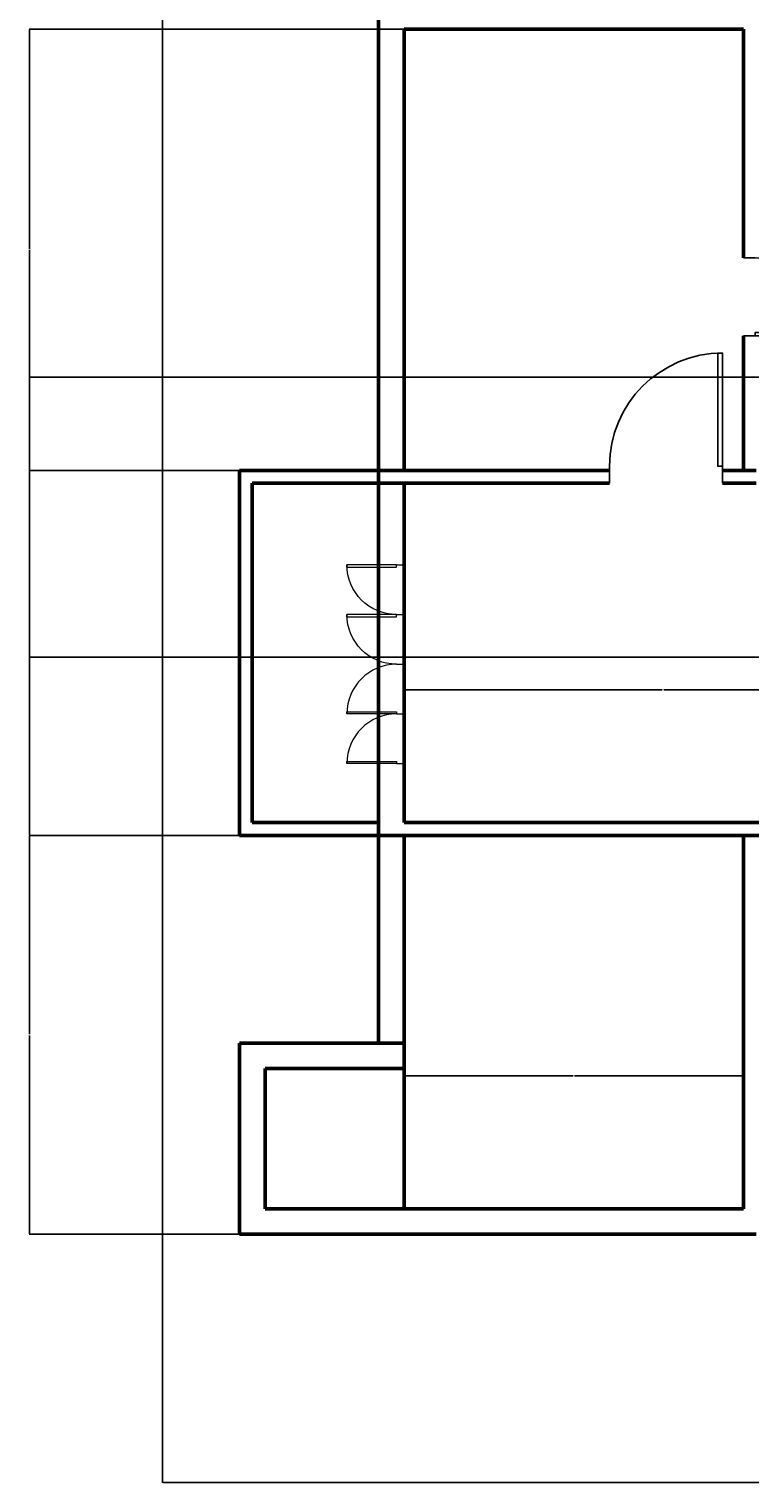
# Model space of a CAD drawing. Units: inches. Extents: x 2032 to 3981, y 840 to 2177.
# Tile 1 of 6: x 2032 to 2286, y 840 to 1354. Entities that reach past the tile are written whole.
import ezdxf

# ---------------------------------------------------------------- set-up
doc = ezdxf.new("R2010")
doc.units = ezdxf.units.IN
for name, color, linetype, lineweight in [('A-ANNO-DIMS', 2, 'Continuous', 18), ('A-DOOR', 3, 'Continuous', 25), ('A-GLAZ', 4, 'Continuous', 18), ('A-WALL', 7, 'Continuous', 50)]:
    doc.layers.add(name, color=color, linetype=linetype, lineweight=lineweight)
doc.styles.get("Standard").update_dxf_attribs({"font": 'arial.ttf'})
doc.dimstyles.get("Standard").update_dxf_attribs({"dimtxt": 0.18, "dimasz": 0.18, "dimexe": 0.18, "dimexo": 0.0625, "dimgap": 0.09, "dimtad": 0, "dimtih": 1, "dimtoh": 1, "dimdec": 4, "dimzin": 0, "dimdsep": 46, "dimtxsty": 'Standard', "dimcen": 0.09, "dimadec": 0, "dimazin": 0, "dimtfac": 1, "dimtdec": 4, "dimtofl": 0, "dimtmove": 0, "dimatfit": 3, "dimfxl": 1, "dimtolj": 1, "dimtzin": 0, "dimarcsym": 0})

# ---------------------------------------------------------------- blocks, each defined once
blk = doc.blocks.new('*U2')
for p, q in [((0, 0), (0, -6)), ((40, 0), (40, -6))]:
    blk.add_line(p, q)
blk.add_lwpolyline([(0, 0), (0, 40), (1.75, 40), (1.75, 0)], close=True)
blk.add_arc((0, 0), 40, 0, 90)
blk = doc.blocks.new('*D14')
at = {"layer": 'A-ANNO-DIMS', "color": 0, "lineweight": -2, "transparency": 16777216}
for p, q in [((2078.89, 1518.9), (2078.89, 840.08)), ((2677.35, 1476.9), (2677.35, 840.08)), ((2079.07, 840.26), (2377.73, 840.26)), ((2677.17, 840.26), (2378.52, 840.26))]:
    blk.add_line(p, q, dxfattribs=at)
at = {"layer": 'A-ANNO-DIMS', "color": 0, "lineweight": 100, "transparency": 16777216}
for points in [[(2079.07, 840.29), (2079.07, 840.23), (2078.89, 840.26)], [(2677.17, 840.29), (2677.17, 840.23), (2677.35, 840.26)]]:
    blk.add_solid(points, dxfattribs=at)
at = {"layer": 'Defpoints', "color": 0, "lineweight": 100, "transparency": 16777216}
for p in [(2078.89, 1518.96), (2677.35, 1476.96), (2677.35, 840.26)]:
    blk.add_point(p, dxfattribs=at)
at = {"layer": 'A-ANNO-DIMS', "color": 0, "transparency": 16777216, "insert": (2378.12, 840.26), "char_height": 0.18, "attachment_point": 5}
blk.add_mtext('\\A1;598.5', dxfattribs=at)
blk = doc.blocks.new('*D22')
at = {"layer": 'A-ANNO-DIMS', "color": 0, "lineweight": -2, "transparency": 16777216}
for p, q in [((2106.03, 1068.96), (2031.71, 1068.96)), ((2031.89, 1068.78), (2031.89, 998.64)), ((2031.89, 928.14), (2031.89, 998.28)), ((2106.03, 927.96), (2031.71, 927.96))]:
    blk.add_line(p, q, dxfattribs=at)
at = {"layer": 'A-ANNO-DIMS', "color": 0, "lineweight": 100, "transparency": 16777216}
for points in [[(2031.86, 1068.78), (2031.92, 1068.78), (2031.89, 1068.96)], [(2031.86, 928.14), (2031.92, 928.14), (2031.89, 927.96)]]:
    blk.add_solid(points, dxfattribs=at)
at = {"layer": 'Defpoints', "color": 0, "lineweight": 100, "transparency": 16777216}
for p in [(2031.89, 1068.96), (2106.09, 1068.96), (2106.09, 927.96)]:
    blk.add_point(p, dxfattribs=at)
at = {"layer": 'A-ANNO-DIMS', "color": 0, "transparency": 16777216, "insert": (2031.89, 998.46), "char_height": 0.18, "attachment_point": 5}
blk.add_mtext('\\A1;141', dxfattribs=at)
blk = doc.blocks.new('*D23')
at = {"layer": 'A-ANNO-DIMS', "color": 0, "lineweight": -2, "transparency": 16777216}
for p, q in [((2106.03, 1197.96), (2031.71, 1197.96)), ((2031.89, 1197.78), (2031.89, 1133.64)), ((2031.89, 1069.14), (2031.89, 1133.28)), ((2106.03, 1068.96), (2031.71, 1068.96))]:
    blk.add_line(p, q, dxfattribs=at)
at = {"layer": 'A-ANNO-DIMS', "color": 0, "lineweight": 100, "transparency": 16777216}
for points in [[(2031.86, 1197.78), (2031.92, 1197.78), (2031.89, 1197.96)], [(2031.86, 1069.14), (2031.92, 1069.14), (2031.89, 1068.96)]]:
    blk.add_solid(points, dxfattribs=at)
at = {"layer": 'Defpoints', "color": 0, "lineweight": 100, "transparency": 16777216}
for p in [(2031.89, 1197.96), (2106.09, 1197.96), (2106.09, 1068.96)]:
    blk.add_point(p, dxfattribs=at)
at = {"layer": 'A-ANNO-DIMS', "color": 0, "transparency": 16777216, "insert": (2031.89, 1133.46), "char_height": 0.18, "attachment_point": 5}
blk.add_mtext('\\A1;129', dxfattribs=at)
blk = doc.blocks.new('*D24')
at = {"layer": 'A-ANNO-DIMS', "color": 0, "lineweight": -2, "transparency": 16777216}
for p, q in [((2164.15, 1353.96), (2031.71, 1353.96)), ((2031.89, 1353.78), (2031.89, 1276.14)), ((2031.89, 1198.14), (2031.89, 1275.78)), ((2106.03, 1197.96), (2031.71, 1197.96))]:
    blk.add_line(p, q, dxfattribs=at)
at = {"layer": 'A-ANNO-DIMS', "color": 0, "lineweight": 100, "transparency": 16777216}
for points in [[(2031.86, 1353.78), (2031.92, 1353.78), (2031.89, 1353.96)], [(2031.86, 1198.14), (2031.92, 1198.14), (2031.89, 1197.96)]]:
    blk.add_solid(points, dxfattribs=at)
at = {"layer": 'Defpoints', "color": 0, "lineweight": 100, "transparency": 16777216}
for p in [(2031.89, 1353.96), (2164.21, 1353.96), (2106.09, 1197.96)]:
    blk.add_point(p, dxfattribs=at)
at = {"layer": 'A-ANNO-DIMS', "color": 0, "transparency": 16777216, "insert": (2031.89, 1275.96), "char_height": 0.18, "attachment_point": 5}
blk.add_mtext('\\A1;156', dxfattribs=at)
blk = doc.blocks.new('*D44')
at = {"layer": 'A-ANNO-DIMS', "color": 0, "lineweight": -2, "transparency": 16777216}
for p, q in [((2164.21, 1073.52), (2164.21, 1120.64)), ((2164.39, 1120.46), (2255.43, 1120.46)), ((2347.03, 1120.46), (2255.99, 1120.46)), ((2347.21, 1073.52), (2347.21, 1120.64))]:
    blk.add_line(p, q, dxfattribs=at)
at = {"layer": 'A-ANNO-DIMS', "color": 0, "lineweight": 100, "transparency": 16777216}
for points in [[(2164.39, 1120.49), (2164.39, 1120.43), (2164.21, 1120.46)], [(2347.03, 1120.49), (2347.03, 1120.43), (2347.21, 1120.46)]]:
    blk.add_solid(points, dxfattribs=at)
at = {"layer": 'Defpoints', "color": 0, "lineweight": 100, "transparency": 16777216}
for p in [(2347.21, 1120.46), (2164.21, 1073.46), (2347.21, 1073.46)]:
    blk.add_point(p, dxfattribs=at)
at = {"layer": 'A-ANNO-DIMS', "color": 0, "transparency": 16777216, "insert": (2255.71, 1120.46), "char_height": 0.18, "attachment_point": 5}
blk.add_mtext('\\A1;183', dxfattribs=at)
blk = doc.blocks.new('*D45')
at = {"layer": 'A-ANNO-DIMS', "color": 0, "lineweight": -2, "transparency": 16777216}
for p, q in [((2164.21, 937.02), (2164.21, 984.14)), ((2164.39, 983.96), (2223.93, 983.96)), ((2284.03, 983.96), (2224.49, 983.96)), ((2284.21, 937.02), (2284.21, 984.14))]:
    blk.add_line(p, q, dxfattribs=at)
at = {"layer": 'A-ANNO-DIMS', "color": 0, "lineweight": 100, "transparency": 16777216}
for points in [[(2164.39, 983.99), (2164.39, 983.93), (2164.21, 983.96)], [(2284.03, 983.99), (2284.03, 983.93), (2284.21, 983.96)]]:
    blk.add_solid(points, dxfattribs=at)
at = {"layer": 'Defpoints', "color": 0, "lineweight": 100, "transparency": 16777216}
for p in [(2284.21, 983.96), (2164.21, 936.96), (2284.21, 936.96)]:
    blk.add_point(p, dxfattribs=at)
at = {"layer": 'A-ANNO-DIMS', "color": 0, "transparency": 16777216, "insert": (2224.21, 983.96), "char_height": 0.18, "attachment_point": 5}
blk.add_mtext('\\A1;120', dxfattribs=at)
blk = doc.blocks.new('*D58')
at = {"layer": 'A-ANNO-DIMS', "color": 0, "lineweight": -2, "transparency": 16777216}
for p, q in [((2474.87, 1230.96), (2031.71, 1230.96)), ((2031.89, 1230.78), (2031.89, 1181.64)), ((2031.89, 1132.14), (2031.89, 1181.28)), ((2474.87, 1131.96), (2031.71, 1131.96))]:
    blk.add_line(p, q, dxfattribs=at)
at = {"layer": 'A-ANNO-DIMS', "color": 0, "lineweight": 100, "transparency": 16777216}
for points in [[(2031.86, 1230.78), (2031.92, 1230.78), (2031.89, 1230.96)], [(2031.86, 1132.14), (2031.92, 1132.14), (2031.89, 1131.96)]]:
    blk.add_solid(points, dxfattribs=at)
at = {"layer": 'Defpoints', "color": 0, "lineweight": 100, "transparency": 16777216}
for p in [(2474.93, 1230.96), (2031.89, 1131.96), (2474.93, 1131.96)]:
    blk.add_point(p, dxfattribs=at)
at = {"layer": 'A-ANNO-DIMS', "color": 0, "transparency": 16777216, "insert": (2031.89, 1181.46), "char_height": 0.18, "attachment_point": 5}
blk.add_mtext('\\A1;99', dxfattribs=at)

msp = doc.modelspace()

# ---------------------------------------------------------------- linework, layer by layer
at = {"layer": 'A-WALL'}
for p, q in [((2155.2092, 1518.9584), (2155.2092, 1353.9584)), ((2155.2092, 1353.9584), (2155.2092, 1193.4584)), ((2164.2092, 1353.9584), (2284.2092, 1353.9584)), ((2164.2092, 1353.9584), (2164.2092, 1197.9584)), ((2284.2092, 1273.0984), (2284.2092, 1353.9584)), ((2284.2092, 1197.9584), (2284.2092, 1245.5139)), ((2106.0893, 1068.9584), (2106.0893, 1197.9584)), ((2106.0893, 1197.9584), (2181.4087, 1197.9584)), ((2164.2092, 1197.9584), (2236.813, 1197.9584)), ((2276.813, 1197.9584), (2284.2092, 1197.9584)), ((2284.2092, 1197.9584), (2288.7092, 1197.9584)), ((2110.5893, 1073.4584), (2110.5893, 1193.4584)), ((2110.5893, 1193.4584), (2181.4087, 1193.4584)), ((2155.2092, 1193.4584), (2236.813, 1193.4584)), ((2155.2092, 1193.4584), (2155.2092, 1068.9584)), ((2164.2092, 1193.4584), (2164.2092, 1073.4584)), ((2276.813, 1193.4584), (2288.7092, 1193.4584)), ((2115.0893, 1068.9584), (2106.0893, 1068.9584)), ((2155.2092, 1073.4584), (2110.5893, 1073.4584)), ((2155.2092, 1068.9584), (2115.0893, 1068.9584)), ((2155.2092, 1068.9584), (2347.2092, 1068.9584)), ((2155.2092, 1068.9584), (2155.2092, 995.5055)), ((2164.2092, 1073.4584), (2347.2092, 1073.4584)), ((2164.2092, 1068.9584), (2164.2092, 936.9584)), ((2284.2092, 936.9584), (2284.2092, 1068.9584)), ((2106.0893, 927.9584), (2106.0893, 995.5055)), ((2106.0893, 995.5055), (2164.2092, 995.5055)), ((2115.0893, 936.9584), (2115.0893, 986.5055)), ((2115.0893, 986.5055), (2164.2092, 986.5055)), ((2164.2092, 936.9584), (2115.0893, 936.9584)), ((2164.2092, 936.9584), (2284.2092, 936.9584)), ((2155.2092, 927.9584), (2106.0893, 927.9584)), ((2155.2092, 927.9584), (2288.7092, 927.9584))]:
    msp.add_line(p, q, dxfattribs=at)

# ---------------------------------------------------------------- block references
at = {"layer": 'A-DOOR', "xscale": -0.6896122567198519, "yscale": 0.6896122567198519, "zscale": 0.6896122567198519, "rotation": 270}
msp.add_blockref('*U2', (2288.3469, 1245.5139), dxfattribs=at)
at = {"layer": 'A-DOOR', "xscale": -1}
msp.add_blockref('*U2', (2276.813, 1199.4584), dxfattribs=at)
at = {"layer": 'A-GLAZ', "yscale": 0.4390204122695697, "zscale": 0.4390204122695697, "rotation": 90}
for p, xscale in [((2161.5751, 1164.5744), -0.4390204122695697), ((2161.5751, 1147.0135), -0.4390204122695697), ((2161.5751, 1111.8919), 0.4390204122695697), ((2161.5751, 1094.3311), 0.4390204122695697)]:
    msp.add_blockref('*U2', p, dxfattribs=dict(at, xscale=xscale))

# ---------------------------------------------------------------- dimensions: what is measured, and where the dimension line sits
at = {"layer": 'A-ANNO-DIMS'}
for base, p1, p2, override, picture, middle in [((2677.3537, 840.2551), (2078.8911, 1518.9584), (2677.3537, 1476.9584), {"dimdec": 1, "dimlfac": 1, "dimrnd": 0, "dimzin": 0, "dimdsep": 46, "dimlunit": 2}, '*D14', (2378.1224, 840.2551)), ((2347.2092, 1120.4584), (2164.2092, 1073.4584), (2347.2092, 1073.4584), {"dimdec": 0, "dimlfac": 1, "dimrnd": 0, "dimzin": 0, "dimdsep": 46, "dimlunit": 2}, '*D44', (2255.7092, 1120.4584)), ((2284.2092, 983.9584), (2164.2092, 936.9584), (2284.2092, 936.9584), {"dimdec": 0, "dimlfac": 1, "dimrnd": 0, "dimzin": 0, "dimdsep": 46, "dimlunit": 2}, '*D45', (2224.2092, 983.9584))]:
    dim = msp.add_linear_dim(base=base, p1=p1, p2=p2, dimstyle='Standard', override=override, dxfattribs=at)
    dim.commit()
    dim.dimension.update_dxf_attribs({"geometry": picture, "text_midpoint": middle})
for base, p1, p2, picture, middle in [((2031.8911, 1353.9584), (2106.0893, 1197.9584), (2164.2092, 1353.9584), '*D24', (2031.8911, 1275.9584)), ((2031.8911, 1131.9584), (2474.9346, 1230.9584), (2474.9346, 1131.9584), '*D58', (2031.8911, 1181.4584)), ((2031.8911, 1197.9584), (2106.0893, 1068.9584), (2106.0893, 1197.9584), '*D23', (2031.8911, 1133.4584)), ((2031.8911, 1068.9584), (2106.0893, 927.9584), (2106.0893, 1068.9584), '*D22', (2031.8911, 998.4584))]:
    dim = msp.add_linear_dim(base=base, p1=p1, p2=p2, angle=90, dimstyle='Standard', override={"dimdec": 0, "dimlfac": 1, "dimrnd": 0, "dimzin": 0, "dimdsep": 46, "dimlunit": 2}, dxfattribs=at)
    dim.commit()
    dim.dimension.update_dxf_attribs({"geometry": picture, "text_midpoint": middle})

doc.saveas('drawing.dxf')
